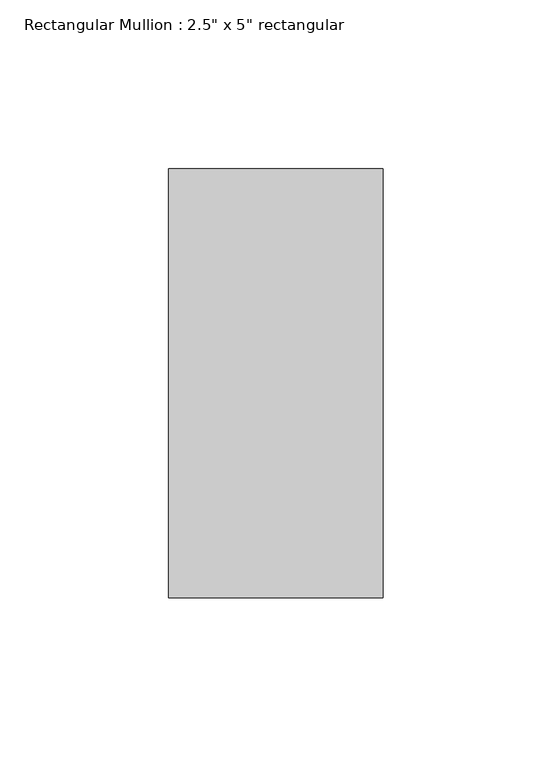
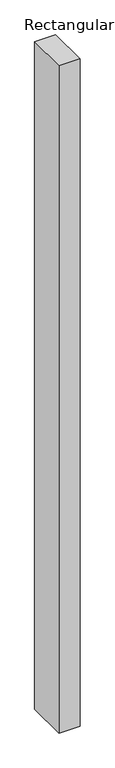
"""IFC4 building model written with IfcOpenShell, lengths in millimetres: member geometry."""

from ifc_helpers import new_model, si_unit, frame, origin, place, context, project, spatial, polyline, outline, extrude, source, transform, mapped, element, save


def member_7cbddb58(model_context):
    return source(origin(), model_context, "Body", "SweptSolid", [
        extrude(outline(polyline([(31.75, 63.5), (31.75, -63.5), (-31.75, -63.5), (-31.75, 63.5), (31.75, 63.5)])), frame((0.0, 0.0, -2133.6), z_axis=(0.0, 0.0, 1.0), x_axis=(1.0, 0.0, 0.0)), (0.0, 0.0, 1.0), 2133.6),
    ])


if __name__ == "__main__":
    model = new_model("IFC4")
    model_context = context("Model", 3, world=origin())
    ifc_project = project(units=[si_unit("LENGTHUNIT", "METRE", prefix="MILLI")], contexts=[model_context])
    site = spatial("IfcSite", under=ifc_project)
    building = spatial("IfcBuilding", under=site)
    placement = place(None, origin())
    member_shape = member_7cbddb58(model_context)
    element("IfcMember", 1, ObjectType="Rectangular Mullion : 2.5\" x 5\" rectangular", at=placement, inside=building, context=model_context, shape_type="MappedRepresentation", body=[
        mapped(member_shape, transform((0.0, 0.0, 0.0), x_axis=(1.0, 0.0, 0.0), y_axis=(0.0, 1.0, 0.0), z_axis=(0.0, 0.0, 1.0))),
    ])
    save(model, "model.ifc")

# Revit data of these elements
# Type "Rectangular Mullion : 2.5\" x 5\" rectangular"
#   built-in parameter 1007304 = 0.416667 (stored number, unit not read)
#   built-in parameter 1007301 = 0.104167 (stored number, unit not read)
#   built-in parameter 1007300 = 0.104167 (stored number, unit not read)
